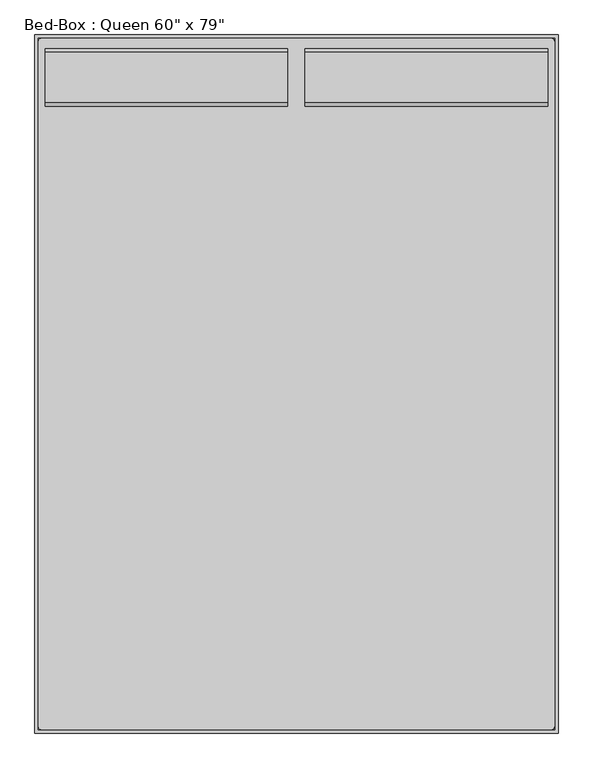
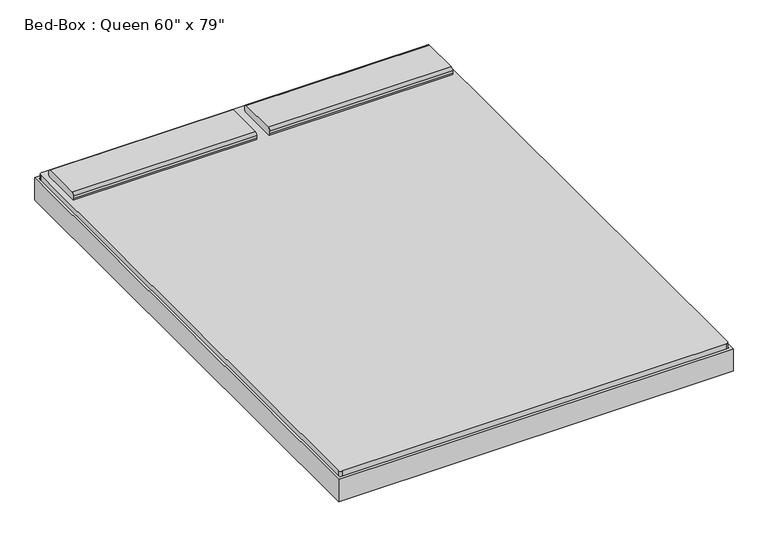
"""IFC4 building model written with IfcOpenShell, lengths in millimetres: furniture geometry."""

from ifc_helpers import new_model, si_unit, point, frame, frame_2d, origin, place, context, project, spatial, polyline, circle_curve, trimmed, segment, composite_curve, outline, extrude, source, transform, mapped, element, save
from ifc_brep_helpers import plane_surface, cylinder_surface, revolved_surface, advanced_brep


def furniture_0647d374(model_context):
    return source(origin(), model_context, "Body", "SolidModel", [
        advanced_brep(
        [(-1540.447541, -2469.6295082, 196.85), (-1540.447541, -2469.6295082, 177.8), (-1540.447541, -2545.8295082, 177.8), (-1540.447541, -2545.8295082, 196.85), (-1477.5113525, -2469.6295082, 196.85), (-1489.647541, -2469.6295082, 177.8), (-1489.647541, -2545.8295082, 177.8), (-1477.5113525, -2545.8295082, 196.85), (-1396.3115092, -2469.6295082, 22.716374), (-1413.5766725, -2469.6295082, 14.6654962), (-1413.5766725, -2545.8295082, 14.6654962), (-1396.3115092, -2545.8295082, 22.716374), (-1390.5564547, -2469.6295082, 0.0), (-1390.5564547, -2469.6295082, 19.05), (-1390.5564547, -2545.8295082, 0.0), (-1390.5564547, -2545.8295082, 19.05), (-1311.9439489, -2469.6295082, 19.05), (-1311.9439489, -2469.6295082, 0.0), (-1311.9439489, -2545.8295082, 0.0), (-1311.9439489, -2545.8295082, 19.05), (-1299.2439489, -2469.6295082, 3.4029547), (-1308.7689489, -2469.6295082, 19.9007387), (-1299.2439489, -2545.8295082, 3.4029547), (-1308.7689489, -2545.8295082, 19.9007387), (-1244.2513357, -2469.6295082, 57.15), (-1239.1469036, -2469.6295082, 38.1), (-1239.1469036, -2545.8295082, 38.1), (-1244.2513357, -2545.8295082, 57.15), (1922.5562537, -2469.6295082, 57.15), (1917.4518216, -2469.6295082, 38.1), (1917.4518216, -2545.8295082, 38.1), (1922.5562537, -2545.8295082, 57.15), (1987.0738669, -2469.6295082, 19.9007387), (1977.5488669, -2469.6295082, 3.4029547), (1977.5488669, -2545.8295082, 3.4029547), (1987.0738669, -2545.8295082, 19.9007387), (1990.2488669, -2469.6295082, 0.0), (1990.2488669, -2469.6295082, 19.05), (1990.2488669, -2545.8295082, 0.0), (1990.2488669, -2545.8295082, 19.05), (2068.8613728, -2469.6295082, 19.05), (2068.8613728, -2469.6295082, 0.0), (2068.8613728, -2545.8295082, 0.0), (2068.8613728, -2545.8295082, 19.05), (2091.8815906, -2469.6295082, 14.6654962), (2074.6164272, -2469.6295082, 22.716374), (2091.8815906, -2545.8295082, 14.6654962), (2074.6164272, -2545.8295082, 22.716374), (2155.8162705, -2469.6295082, 196.85), (2167.952459, -2469.6295082, 177.8), (2167.952459, -2545.8295082, 177.8), (2155.8162705, -2545.8295082, 196.85), (2218.752459, -2469.6295082, 196.85), (2218.752459, -2545.8295082, 196.85), (2218.752459, -2545.8295082, 177.8), (2218.752459, -2469.6295082, 177.8)],
        [
            (0, 1),
            (1, 2),
            (2, 3),
            (3, 0),
            (0, 4),
            (4, 5),
            (5, 1),
            (5, 6),
            (6, 2),
            (6, 7),
            (7, 3),
            (7, 4),
            (4, 8),
            (8, 9),
            (9, 5),
            (9, 10),
            (10, 6),
            (10, 11),
            (11, 7),
            (11, 8),
            (12, 9, circle_curve(frame((-1390.5564547, -2469.6295082, 25.4), z_axis=(0.0, 1.0, 0.0), x_axis=(-0.906307787036663, 0.0, -0.4226182617406713)), 25.4)),
            (8, 13, circle_curve(frame((-1390.5564547, -2469.6295082, 25.4), z_axis=(0.0, -1.0, 0.0), x_axis=(-0.906307787036663, 0.0, -0.4226182617406713)), 6.35)),
            (13, 12),
            (14, 10, circle_curve(frame((-1390.5564547, -2545.8295082, 25.4), z_axis=(0.0, 1.0, 0.0), x_axis=(-0.906307787036663, 0.0, -0.4226182617406713)), 25.4)),
            (12, 14),
            (15, 11, circle_curve(frame((-1390.5564547, -2545.8295082, 25.4), z_axis=(0.0, 1.0, 0.0), x_axis=(-0.906307787036663, 0.0, -0.4226182617406713)), 6.35)),
            (14, 15),
            (15, 13),
            (13, 16),
            (16, 17),
            (17, 12),
            (17, 18),
            (18, 14),
            (18, 19),
            (19, 15),
            (19, 16),
            (20, 17, circle_curve(frame((-1311.9439489, -2469.6295082, 25.4), z_axis=(0.0, 1.0, 0.0), x_axis=(0.0, 0.0, -1.0)), 25.4)),
            (16, 21, circle_curve(frame((-1311.9439489, -2469.6295082, 25.4), z_axis=(0.0, -1.0, 0.0), x_axis=(0.0, 0.0, -1.0)), 6.35)),
            (21, 20),
            (22, 18, circle_curve(frame((-1311.9439489, -2545.8295082, 25.4), z_axis=(0.0, 1.0, 0.0), x_axis=(0.0, 0.0, -1.0)), 25.4)),
            (20, 22),
            (23, 19, circle_curve(frame((-1311.9439489, -2545.8295082, 25.4), z_axis=(0.0, 1.0, 0.0), x_axis=(0.0, 0.0, -1.0)), 6.35)),
            (22, 23),
            (23, 21),
            (21, 24),
            (24, 25),
            (25, 20),
            (25, 26),
            (26, 22),
            (26, 27),
            (27, 23),
            (27, 24),
            (24, 28),
            (28, 29),
            (29, 25),
            (29, 30),
            (30, 26),
            (30, 31),
            (31, 27),
            (31, 28),
            (28, 32),
            (32, 33),
            (33, 29),
            (33, 34),
            (34, 30),
            (34, 35),
            (35, 31),
            (35, 32),
            (36, 33, circle_curve(frame((1990.2488669, -2469.6295082, 25.4), z_axis=(0.0, 1.0, 0.0), x_axis=(-0.5000000000000479, 0.0, -0.866025403784411)), 25.4)),
            (32, 37, circle_curve(frame((1990.2488669, -2469.6295082, 25.4), z_axis=(0.0, -1.0, 0.0), x_axis=(-0.5000000000000479, 0.0, -0.866025403784411)), 6.35)),
            (37, 36),
            (38, 34, circle_curve(frame((1990.2488669, -2545.8295082, 25.4), z_axis=(0.0, 1.0, 0.0), x_axis=(-0.5000000000000479, 0.0, -0.866025403784411)), 25.4)),
            (36, 38),
            (39, 35, circle_curve(frame((1990.2488669, -2545.8295082, 25.4), z_axis=(0.0, 1.0, 0.0), x_axis=(-0.5000000000000479, 0.0, -0.866025403784411)), 6.35)),
            (38, 39),
            (39, 37),
            (37, 40),
            (40, 41),
            (41, 36),
            (41, 42),
            (42, 38),
            (42, 43),
            (43, 39),
            (43, 40),
            (44, 41, circle_curve(frame((2068.8613728, -2469.6295082, 25.4), z_axis=(0.0, 1.0, 0.0), x_axis=(0.0, 0.0, -1.0)), 25.4)),
            (40, 45, circle_curve(frame((2068.8613728, -2469.6295082, 25.4), z_axis=(0.0, -1.0, 0.0), x_axis=(0.0, 0.0, -1.0)), 6.35)),
            (45, 44),
            (46, 42, circle_curve(frame((2068.8613728, -2545.8295082, 25.4), z_axis=(0.0, 1.0, 0.0), x_axis=(0.0, 0.0, -1.0)), 25.4)),
            (44, 46),
            (47, 43, circle_curve(frame((2068.8613728, -2545.8295082, 25.4), z_axis=(0.0, 1.0, 0.0), x_axis=(0.0, 0.0, -1.0)), 6.35)),
            (46, 47),
            (47, 45),
            (45, 48),
            (48, 49),
            (49, 44),
            (49, 50),
            (50, 46),
            (50, 51),
            (51, 47),
            (51, 48),
            (52, 53),
            (53, 54),
            (54, 55),
            (55, 52),
            (48, 52),
            (55, 49),
            (54, 50),
            (53, 51),
        ],
        [
            plane_surface(frame((-1540.447541, -2774.4295082, -127.5947323), z_axis=(-1.0, 0.0, 0.0), x_axis=(0.0, 1.0, 0.0))),
            plane_surface(frame((-1540.447541, -2469.6295082, 196.85), z_axis=(0.0, 1.0, 0.0), x_axis=(1.0, 0.0, 0.0))),
            plane_surface(frame((-1540.447541, -2469.6295082, 177.8), z_axis=(0.0, 0.0, -1.0), x_axis=(1.0, 0.0, 0.0))),
            plane_surface(frame((-1540.447541, -2545.8295082, 177.8), z_axis=(0.0, -1.0, 0.0), x_axis=(1.0, 0.0, 0.0))),
            plane_surface(frame((-1540.447541, -2545.8295082, 196.85), z_axis=(0.0, 0.0, 1.0), x_axis=(1.0, 0.0, 0.0))),
            plane_surface(frame((-1477.5113525, -2469.6295082, 196.85), z_axis=(0.0, 1.0, 0.0), x_axis=(0.42261826174067096, 0.0, -0.9063077870366633))),
            plane_surface(frame((-1489.647541, -2469.6295082, 177.8), z_axis=(-0.9063077870366629, 0.0, -0.4226182617406717), x_axis=(0.4226182617406717, 0.0, -0.9063077870366629))),
            plane_surface(frame((-1489.647541, -2545.8295082, 177.8), z_axis=(0.0, -1.0, 0.0), x_axis=(0.4226182617406704, 0.0, -0.9063077870366635))),
            plane_surface(frame((-1477.5113525, -2545.8295082, 196.85), z_axis=(0.906307787036663, 0.0, 0.42261826174067146), x_axis=(0.42261826174067146, 0.0, -0.906307787036663))),
            plane_surface(frame((-1390.5564547, -2469.6295082, 25.4), z_axis=(0.0, 1.0, 0.0), x_axis=(-0.906307787036663, 0.0, -0.4226182617406713))),
            cylinder_surface(frame((-1390.5564547, -2774.4295082, 25.4), z_axis=(0.0, -1.0, 0.0), x_axis=(-0.906307787036663, 0.0, -0.4226182617406713)), 25.4),
            plane_surface(frame((-1390.5564547, -2545.8295082, 25.4), z_axis=(0.0, -1.0, 0.0), x_axis=(-0.906307787036663, 0.0, -0.4226182617406713))),
            revolved_surface(polyline([(-1396.3115091476827, -2545.8295082, 22.716374037946736), (-1396.3115091476827, -2469.6295082, 22.716374037946736)]), (-1390.5564547, -2774.4295082, 25.4), (0.0, -1.0, 0.0)),
            plane_surface(frame((-1390.5564547, -2469.6295082, 19.05), z_axis=(0.0, 1.0, 0.0), x_axis=(1.0, 0.0, 0.0))),
            plane_surface(frame((-1390.5564547, -2469.6295082, 0.0), z_axis=(0.0, 0.0, -1.0), x_axis=(1.0, 0.0, 0.0))),
            plane_surface(frame((-1390.5564547, -2545.8295082, 0.0), z_axis=(0.0, -1.0, 0.0), x_axis=(1.0, 0.0, 0.0))),
            plane_surface(frame((-1390.5564547, -2545.8295082, 19.05), z_axis=(0.0, 0.0, 1.0), x_axis=(1.0, 0.0, 0.0))),
            plane_surface(frame((-1311.9439489, -2469.6295082, 25.4), z_axis=(0.0, 1.0, 0.0), x_axis=(0.0, 0.0, -1.0))),
            cylinder_surface(frame((-1311.9439489, -2774.4295082, 25.4), z_axis=(0.0, -1.0, 0.0), x_axis=(0.0, 0.0, -1.0)), 25.4),
            plane_surface(frame((-1311.9439489, -2545.8295082, 25.4), z_axis=(0.0, -1.0, 0.0), x_axis=(0.0, 0.0, -1.0))),
            revolved_surface(polyline([(-1311.9439489, -2545.8295082, 19.049999999999997), (-1311.9439489, -2469.6295082, 19.049999999999997)]), (-1311.9439489, -2774.4295082, 25.4), (0.0, -1.0, 0.0)),
            plane_surface(frame((-1308.7689489, -2469.6295082, 19.9007387), z_axis=(0.0, 1.0000000000000002, 0.0), x_axis=(0.8660254037844785, 0.0, 0.4999999999999312))),
            plane_surface(frame((-1299.2439489, -2469.6295082, 3.4029547), z_axis=(0.49999999999993033, 0.0, -0.8660254037844789), x_axis=(0.8660254037844789, 0.0, 0.49999999999993033))),
            plane_surface(frame((-1299.2439489, -2545.8295082, 3.4029547), z_axis=(0.0, -1.0, 0.0), x_axis=(0.8660254037844797, 0.0, 0.4999999999999289))),
            plane_surface(frame((-1308.7689489, -2545.8295082, 19.9007387), z_axis=(-0.4999999999999325, 0.0, 0.8660254037844777), x_axis=(0.8660254037844777, 0.0, 0.4999999999999325))),
            plane_surface(frame((-1244.2513357, -2469.6295082, 57.15), z_axis=(0.0, 1.0, 0.0), x_axis=(1.0, 0.0, 0.0))),
            plane_surface(frame((-1239.1469036, -2469.6295082, 38.1), z_axis=(0.0, 0.0, -1.0), x_axis=(1.0, 0.0, 0.0))),
            plane_surface(frame((-1239.1469036, -2545.8295082, 38.1), z_axis=(0.0, -1.0, 0.0), x_axis=(1.0, 0.0, 0.0))),
            plane_surface(frame((-1244.2513357, -2545.8295082, 57.15), z_axis=(0.0, 0.0, 1.0), x_axis=(1.0, 0.0, 0.0))),
            plane_surface(frame((1922.5562537, -2469.6295082, 57.15), z_axis=(0.0, 1.0, 0.0), x_axis=(0.86602540378441, 0.0, -0.5000000000000497))),
            plane_surface(frame((1917.4518216, -2469.6295082, 38.1), z_axis=(-0.5000000000000524, 0.0, -0.8660254037844084), x_axis=(0.8660254037844084, 0.0, -0.5000000000000524))),
            plane_surface(frame((1917.4518216, -2545.8295082, 38.1), z_axis=(0.0, -1.0, 0.0), x_axis=(0.8660254037844108, 0.0, -0.5000000000000483))),
            plane_surface(frame((1922.5562537, -2545.8295082, 57.15), z_axis=(0.500000000000048, 0.0, 0.866025403784411), x_axis=(0.866025403784411, 0.0, -0.500000000000048))),
            plane_surface(frame((1990.2488669, -2469.6295082, 25.4), z_axis=(0.0, 1.0000000000000002, 0.0), x_axis=(-0.500000000000048, 0.0, -0.8660254037844111))),
            cylinder_surface(frame((1990.2488669, -2774.4295082, 25.4), z_axis=(0.0, -1.0, 0.0), x_axis=(-0.5000000000000479, 0.0, -0.866025403784411)), 25.4),
            plane_surface(frame((1990.2488669, -2545.8295082, 25.4), z_axis=(0.0, -1.0000000000000002, 0.0), x_axis=(-0.500000000000048, 0.0, -0.8660254037844111))),
            revolved_surface(polyline([(1987.0738668999995, -2545.8295082, 19.90073868596899), (1987.0738668999995, -2469.6295082, 19.90073868596899)]), (1990.2488669, -2774.4295082, 25.4), (0.0, -1.0, 0.0)),
            plane_surface(frame((1990.2488669, -2469.6295082, 19.05), z_axis=(0.0, 1.0, 0.0), x_axis=(1.0, 0.0, 0.0))),
            plane_surface(frame((1990.2488669, -2469.6295082, 0.0), z_axis=(0.0, 0.0, -1.0), x_axis=(1.0, 0.0, 0.0))),
            plane_surface(frame((1990.2488669, -2545.8295082, 0.0), z_axis=(0.0, -1.0, 0.0), x_axis=(1.0, 0.0, 0.0))),
            plane_surface(frame((1990.2488669, -2545.8295082, 19.05), z_axis=(0.0, 0.0, 1.0), x_axis=(1.0, 0.0, 0.0))),
            plane_surface(frame((2068.8613728, -2469.6295082, 25.4), z_axis=(0.0, 1.0, 0.0), x_axis=(0.0, 0.0, -1.0))),
            cylinder_surface(frame((2068.8613728, -2774.4295082, 25.4), z_axis=(0.0, -1.0, 0.0), x_axis=(0.0, 0.0, -1.0)), 25.4),
            plane_surface(frame((2068.8613728, -2545.8295082, 25.4), z_axis=(0.0, -1.0, 0.0), x_axis=(0.0, 0.0, -1.0))),
            revolved_surface(polyline([(2068.8613728, -2545.8295082, 19.049999999999997), (2068.8613728, -2469.6295082, 19.049999999999997)]), (2068.8613728, -2774.4295082, 25.4), (0.0, -1.0, 0.0)),
            plane_surface(frame((2074.6164272, -2469.6295082, 22.716374), z_axis=(0.0, 1.0, 0.0), x_axis=(0.4226182617405407, 0.0, 0.906307787036724))),
            plane_surface(frame((2091.8815906, -2469.6295082, 14.6654962), z_axis=(0.9063077870367238, 0.0, -0.4226182617405412), x_axis=(0.4226182617405412, 0.0, 0.9063077870367238))),
            plane_surface(frame((2091.8815906, -2545.8295082, 14.6654962), z_axis=(0.0, -1.0000000000000002, 0.0), x_axis=(0.422618261740542, 0.0, 0.9063077870367234))),
            plane_surface(frame((2074.6164272, -2545.8295082, 22.716374), z_axis=(-0.9063077870367237, 0.0, 0.4226182617405417), x_axis=(0.4226182617405417, 0.0, 0.9063077870367237))),
            plane_surface(frame((2218.752459, -2774.4295082, -127.5947323), z_axis=(1.0, 0.0, 0.0), x_axis=(0.0, 1.0, 0.0))),
            plane_surface(frame((2155.8162705, -2469.6295082, 196.85), z_axis=(0.0, 1.0, 0.0), x_axis=(1.0, 0.0, 0.0))),
            plane_surface(frame((2167.952459, -2469.6295082, 177.8), z_axis=(0.0, 0.0, -1.0), x_axis=(1.0, 0.0, 0.0))),
            plane_surface(frame((2167.952459, -2545.8295082, 177.8), z_axis=(0.0, -1.0, 0.0), x_axis=(1.0, 0.0, 0.0))),
            plane_surface(frame((2155.8162705, -2545.8295082, 196.85), z_axis=(0.0, 0.0, 1.0), x_axis=(1.0, 0.0, 0.0))),
        ],
        [
            (0, [[1, 2, 3, 4]]),
            (1, [[-1, 5, 6, 7]]),
            (2, [[-2, -7, 8, 9]]),
            (3, [[-3, -9, 10, 11]]),
            (4, [[-4, -11, 12, -5]]),
            (5, [[-6, 13, 14, 15]]),
            (6, [[-8, -15, 16, 17]]),
            (7, [[-10, -17, 18, 19]]),
            (8, [[-12, -19, 20, -13]]),
            (9, [[21, -14, 22, 23]]),
            (10, [[24, -16, -21, 25]]),
            (11, [[26, -18, -24, 27]]),
            (12, [[-22, -20, -26, 28]]),
            (13, [[-23, 29, 30, 31]]),
            (14, [[-25, -31, 32, 33]]),
            (15, [[-27, -33, 34, 35]]),
            (16, [[-28, -35, 36, -29]]),
            (17, [[37, -30, 38, 39]]),
            (18, [[40, -32, -37, 41]]),
            (19, [[42, -34, -40, 43]]),
            (20, [[-38, -36, -42, 44]]),
            (21, [[-39, 45, 46, 47]]),
            (22, [[-41, -47, 48, 49]]),
            (23, [[-43, -49, 50, 51]]),
            (24, [[-44, -51, 52, -45]]),
            (25, [[-46, 53, 54, 55]]),
            (26, [[-48, -55, 56, 57]]),
            (27, [[-50, -57, 58, 59]]),
            (28, [[-52, -59, 60, -53]]),
            (29, [[-54, 61, 62, 63]]),
            (30, [[-56, -63, 64, 65]]),
            (31, [[-58, -65, 66, 67]]),
            (32, [[-60, -67, 68, -61]]),
            (33, [[69, -62, 70, 71]]),
            (34, [[72, -64, -69, 73]]),
            (35, [[74, -66, -72, 75]]),
            (36, [[-70, -68, -74, 76]]),
            (37, [[-71, 77, 78, 79]]),
            (38, [[-73, -79, 80, 81]]),
            (39, [[-75, -81, 82, 83]]),
            (40, [[-76, -83, 84, -77]]),
            (41, [[85, -78, 86, 87]]),
            (42, [[88, -80, -85, 89]]),
            (43, [[90, -82, -88, 91]]),
            (44, [[-86, -84, -90, 92]]),
            (45, [[-87, 93, 94, 95]]),
            (46, [[-89, -95, 96, 97]]),
            (47, [[-91, -97, 98, 99]]),
            (48, [[-92, -99, 100, -93]]),
            (49, [[101, 102, 103, 104]]),
            (50, [[-94, 105, -104, 106]]),
            (51, [[-96, -106, -103, 107]]),
            (52, [[-98, -107, -102, 108]]),
            (53, [[-100, -108, -101, -105]]),
        ],
    ),
        extrude(outline(composite_curve([segment(polyline([(-1515.047541, 2280.1704918), (2193.352459, 2280.1704918)]), True, "CONTINUOUS"), segment(trimmed(circle_curve(frame_2d((2193.352459, 2254.7704918)), 25.4), [point((2193.352459, 2280.1704918))], [point((2218.752459, 2254.7704918))], False, "CARTESIAN"), True, "CONTINUOUS"), segment(polyline([(2218.752459, 2254.7704918), (2218.752459, -2723.6295082)]), True, "CONTINUOUS"), segment(trimmed(circle_curve(frame_2d((2193.352459, -2723.6295082)), 25.4), [point((2218.752459, -2723.6295082))], [point((2193.352459, -2749.0295082))], False, "CARTESIAN"), True, "CONTINUOUS"), segment(polyline([(2193.352459, -2749.0295082), (-1515.047541, -2749.0295082)]), True, "CONTINUOUS"), segment(trimmed(circle_curve(frame_2d((-1515.047541, -2723.6295082)), 25.4), [point((-1515.047541, -2749.0295082))], [point((-1540.447541, -2723.6295082))], False, "CARTESIAN"), True, "CONTINUOUS"), segment(polyline([(-1540.447541, -2723.6295082), (-1540.447541, 2254.7704918)]), True, "CONTINUOUS"), segment(trimmed(circle_curve(frame_2d((-1515.047541, 2254.7704918)), 25.4), [point((-1540.447541, 2254.7704918))], [point((-1515.047541, 2280.1704918))], False, "CARTESIAN"), True, "CONTINUOUS")], self_intersect=False)), frame((0.0, 0.0, 203.2), z_axis=(0.0, 0.0, 1.0), x_axis=(1.0, 0.0, 0.0)), (0.0, 0.0, 1.0), 203.2),
        advanced_brep(
        [(-1540.1231784, 2051.5704918, 177.8), (-1540.1231784, 1975.3704918, 177.8), (-1540.1231784, 1975.3704918, 196.85), (-1540.1231784, 2051.5704918, 196.85), (-1489.3231784, 2051.5704918, 177.8), (-1489.3231784, 1975.3704918, 177.8), (-1477.1869899, 1975.3704918, 196.85), (-1477.1869899, 2051.5704918, 196.85), (-1413.2523099, 2051.5704918, 14.6654962), (-1413.2523099, 1975.3704918, 14.6654962), (-1395.9871466, 1975.3704918, 22.716374), (-1395.9871466, 2051.5704918, 22.716374), (-1390.2320921, 1975.3704918, 0.0), (-1390.2320921, 2051.5704918, 0.0), (-1390.2320921, 1975.3704918, 19.05), (-1390.2320921, 2051.5704918, 19.05), (-1311.6195862, 2051.5704918, 0.0), (-1311.6195862, 1975.3704918, 0.0), (-1311.6195862, 1975.3704918, 19.05), (-1311.6195862, 2051.5704918, 19.05), (-1298.9195862, 1975.3704918, 3.4029547), (-1298.9195862, 2051.5704918, 3.4029547), (-1308.4445862, 1975.3704918, 19.9007387), (-1308.4445862, 2051.5704918, 19.9007387), (-1238.822541, 2051.5704918, 38.1), (-1238.822541, 1975.3704918, 38.1), (-1243.9269731, 1975.3704918, 57.15), (-1243.9269731, 2051.5704918, 57.15), (1917.4518216, 2051.5704918, 38.1), (1917.4518216, 1975.3704918, 38.1), (1922.5562537, 1975.3704918, 57.15), (1922.5562537, 2051.5704918, 57.15), (1977.5488669, 2051.5704918, 3.4029547), (1977.5488669, 1975.3704918, 3.4029547), (1987.0738669, 1975.3704918, 19.9007387), (1987.0738669, 2051.5704918, 19.9007387), (1990.2488669, 1975.3704918, 0.0), (1990.2488669, 2051.5704918, 0.0), (1990.2488669, 1975.3704918, 19.05), (1990.2488669, 2051.5704918, 19.05), (2068.8613728, 2051.5704918, 0.0), (2068.8613728, 1975.3704918, 0.0), (2068.8613728, 1975.3704918, 19.05), (2068.8613728, 2051.5704918, 19.05), (2091.8815906, 1975.3704918, 14.6654962), (2091.8815906, 2051.5704918, 14.6654962), (2074.6164272, 1975.3704918, 22.716374), (2074.6164272, 2051.5704918, 22.716374), (2167.952459, 2051.5704918, 177.8), (2167.952459, 1975.3704918, 177.8), (2155.8162705, 1975.3704918, 196.85), (2155.8162705, 2051.5704918, 196.85), (2218.752459, 2051.5704918, 177.8), (2218.752459, 2051.5704918, 196.85), (2218.752459, 1975.3704918, 196.85), (2218.752459, 1975.3704918, 177.8)],
        [
            (0, 1),
            (1, 2),
            (2, 3),
            (3, 0),
            (0, 4),
            (4, 5),
            (5, 1),
            (5, 6),
            (6, 2),
            (6, 7),
            (7, 3),
            (7, 4),
            (4, 8),
            (8, 9),
            (9, 5),
            (9, 10),
            (10, 6),
            (10, 11),
            (11, 7),
            (11, 8),
            (12, 9, circle_curve(frame((-1390.2320921, 1975.3704918, 25.4), z_axis=(0.0, 1.0, 0.0), x_axis=(-0.9063077870366486, 0.0, -0.42261826174070233)), 25.4)),
            (8, 13, circle_curve(frame((-1390.2320921, 2051.5704918, 25.4), z_axis=(0.0, -1.0, 0.0), x_axis=(-0.9063077870366486, 0.0, -0.42261826174070233)), 25.4)),
            (13, 12),
            (14, 10, circle_curve(frame((-1390.2320921, 1975.3704918, 25.4), z_axis=(0.0, 1.0, 0.0), x_axis=(-0.9063077870366486, 0.0, -0.42261826174070233)), 6.35)),
            (12, 14),
            (15, 11, circle_curve(frame((-1390.2320921, 2051.5704918, 25.4), z_axis=(0.0, 1.0, 0.0), x_axis=(-0.9063077870366486, 0.0, -0.42261826174070233)), 6.35)),
            (14, 15),
            (15, 13),
            (13, 16),
            (16, 17),
            (17, 12),
            (17, 18),
            (18, 14),
            (18, 19),
            (19, 15),
            (19, 16),
            (20, 17, circle_curve(frame((-1311.6195862, 1975.3704918, 25.4), z_axis=(0.0, 1.0, 0.0), x_axis=(0.0, 0.0, -1.0)), 25.4)),
            (16, 21, circle_curve(frame((-1311.6195862, 2051.5704918, 25.4), z_axis=(0.0, -1.0, 0.0), x_axis=(0.0, 0.0, -1.0)), 25.4)),
            (21, 20),
            (22, 18, circle_curve(frame((-1311.6195862, 1975.3704918, 25.4), z_axis=(0.0, 1.0, 0.0), x_axis=(0.0, 0.0, -1.0)), 6.35)),
            (20, 22),
            (23, 19, circle_curve(frame((-1311.6195862, 2051.5704918, 25.4), z_axis=(0.0, 1.0, 0.0), x_axis=(0.0, 0.0, -1.0)), 6.35)),
            (22, 23),
            (23, 21),
            (21, 24),
            (24, 25),
            (25, 20),
            (25, 26),
            (26, 22),
            (26, 27),
            (27, 23),
            (27, 24),
            (24, 28),
            (28, 29),
            (29, 25),
            (29, 30),
            (30, 26),
            (30, 31),
            (31, 27),
            (31, 28),
            (28, 32),
            (32, 33),
            (33, 29),
            (33, 34),
            (34, 30),
            (34, 35),
            (35, 31),
            (35, 32),
            (36, 33, circle_curve(frame((1990.2488669, 1975.3704918, 25.4), z_axis=(0.0, 1.0, 0.0), x_axis=(-0.5000000000000463, 0.0, -0.8660254037844118)), 25.4)),
            (32, 37, circle_curve(frame((1990.2488669, 2051.5704918, 25.4), z_axis=(0.0, -1.0, 0.0), x_axis=(-0.5000000000000463, 0.0, -0.8660254037844118)), 25.4)),
            (37, 36),
            (38, 34, circle_curve(frame((1990.2488669, 1975.3704918, 25.4), z_axis=(0.0, 1.0, 0.0), x_axis=(-0.5000000000000463, 0.0, -0.8660254037844118)), 6.35)),
            (36, 38),
            (39, 35, circle_curve(frame((1990.2488669, 2051.5704918, 25.4), z_axis=(0.0, 1.0, 0.0), x_axis=(-0.5000000000000463, 0.0, -0.8660254037844118)), 6.35)),
            (38, 39),
            (39, 37),
            (37, 40),
            (40, 41),
            (41, 36),
            (41, 42),
            (42, 38),
            (42, 43),
            (43, 39),
            (43, 40),
            (44, 41, circle_curve(frame((2068.8613728, 1975.3704918, 25.4), z_axis=(0.0, 1.0, 0.0), x_axis=(0.0, 0.0, -1.0)), 25.4)),
            (40, 45, circle_curve(frame((2068.8613728, 2051.5704918, 25.4), z_axis=(0.0, -1.0, 0.0), x_axis=(0.0, 0.0, -1.0)), 25.4)),
            (45, 44),
            (46, 42, circle_curve(frame((2068.8613728, 1975.3704918, 25.4), z_axis=(0.0, 1.0, 0.0), x_axis=(0.0, 0.0, -1.0)), 6.35)),
            (44, 46),
            (47, 43, circle_curve(frame((2068.8613728, 2051.5704918, 25.4), z_axis=(0.0, 1.0, 0.0), x_axis=(0.0, 0.0, -1.0)), 6.35)),
            (46, 47),
            (47, 45),
            (45, 48),
            (48, 49),
            (49, 44),
            (49, 50),
            (50, 46),
            (50, 51),
            (51, 47),
            (51, 48),
            (52, 53),
            (53, 54),
            (54, 55),
            (55, 52),
            (48, 52),
            (55, 49),
            (54, 50),
            (53, 51),
        ],
        [
            plane_surface(frame((-1540.1231784, 2305.5704918, -152.9490627), z_axis=(-1.0, 0.0, 0.0), x_axis=(0.0, 1.0, 0.0))),
            plane_surface(frame((-1540.1231784, 2051.5704918, 177.8), z_axis=(0.0, 0.0, -1.0), x_axis=(1.0, 0.0, 0.0))),
            plane_surface(frame((-1540.1231784, 1975.3704918, 177.8), z_axis=(0.0, -1.0, 0.0), x_axis=(1.0, 0.0, 0.0))),
            plane_surface(frame((-1540.1231784, 1975.3704918, 196.85), z_axis=(0.0, 0.0, 1.0), x_axis=(1.0, 0.0, 0.0))),
            plane_surface(frame((-1540.1231784, 2051.5704918, 196.85), z_axis=(0.0, 1.0, 0.0), x_axis=(1.0, 0.0, 0.0))),
            plane_surface(frame((-1489.3231784, 2051.5704918, 177.8), z_axis=(-0.906307787036649, 0.0, -0.42261826174070155), x_axis=(0.42261826174070155, 0.0, -0.906307787036649))),
            plane_surface(frame((-1489.3231784, 1975.3704918, 177.8), z_axis=(0.0, -1.0, 0.0), x_axis=(0.42261826174070133, 0.0, -0.9063077870366492))),
            plane_surface(frame((-1477.1869899, 1975.3704918, 196.85), z_axis=(0.9063077870366489, 0.0, 0.4226182617407018), x_axis=(0.4226182617407018, 0.0, -0.9063077870366489))),
            plane_surface(frame((-1477.1869899, 2051.5704918, 196.85), z_axis=(0.0, 1.0, 0.0), x_axis=(0.4226182617407019, 0.0, -0.9063077870366488))),
            cylinder_surface(frame((-1390.2320921, 2305.5704918, 25.4), z_axis=(0.0, -1.0, 0.0), x_axis=(-0.9063077870366486, 0.0, -0.42261826174070233)), 25.4),
            plane_surface(frame((-1390.2320921, 1975.3704918, 25.4), z_axis=(0.0, -1.0, 0.0), x_axis=(-0.9063077870366486, 0.0, -0.42261826174070233))),
            revolved_surface(polyline([(-1395.9871465476829, 1975.3704918, 22.71637403794654), (-1395.9871465476829, 2051.5704918, 22.71637403794654)]), (-1390.2320921, 2305.5704918, 25.4), (0.0, -1.0, 0.0)),
            plane_surface(frame((-1390.2320921, 2051.5704918, 25.4), z_axis=(0.0, 1.0, 0.0), x_axis=(-0.9063077870366486, 0.0, -0.42261826174070233))),
            plane_surface(frame((-1390.2320921, 2051.5704918, 0.0), z_axis=(0.0, 0.0, -1.0), x_axis=(1.0, 0.0, 0.0))),
            plane_surface(frame((-1390.2320921, 1975.3704918, 0.0), z_axis=(0.0, -1.0, 0.0), x_axis=(1.0, 0.0, 0.0))),
            plane_surface(frame((-1390.2320921, 1975.3704918, 19.05), z_axis=(0.0, 0.0, 1.0), x_axis=(1.0, 0.0, 0.0))),
            plane_surface(frame((-1390.2320921, 2051.5704918, 19.05), z_axis=(0.0, 1.0, 0.0), x_axis=(1.0, 0.0, 0.0))),
            cylinder_surface(frame((-1311.6195862, 2305.5704918, 25.4), z_axis=(0.0, -1.0, 0.0), x_axis=(0.0, 0.0, -1.0)), 25.4),
            plane_surface(frame((-1311.6195862, 1975.3704918, 25.4), z_axis=(0.0, -1.0, 0.0), x_axis=(0.0, 0.0, -1.0))),
            revolved_surface(polyline([(-1311.6195862, 1975.3704918, 19.049999999999997), (-1311.6195862, 2051.5704918, 19.049999999999997)]), (-1311.6195862, 2305.5704918, 25.4), (0.0, -1.0, 0.0)),
            plane_surface(frame((-1311.6195862, 2051.5704918, 25.4), z_axis=(0.0, 1.0, 0.0), x_axis=(0.0, 0.0, -1.0))),
            plane_surface(frame((-1298.9195862, 2051.5704918, 3.4029547), z_axis=(0.49999999999988004, 0.0, -0.866025403784508), x_axis=(0.866025403784508, 0.0, 0.49999999999988004))),
            plane_surface(frame((-1298.9195862, 1975.3704918, 3.4029547), z_axis=(0.0, -1.0, 0.0), x_axis=(0.8660254037845087, 0.0, 0.4999999999998787))),
            plane_surface(frame((-1308.4445862, 1975.3704918, 19.9007387), z_axis=(-0.49999999999987754, 0.0, 0.8660254037845093), x_axis=(0.8660254037845093, 0.0, 0.49999999999987754))),
            plane_surface(frame((-1308.4445862, 2051.5704918, 19.9007387), z_axis=(0.0, 1.0, 0.0), x_axis=(0.8660254037845093, 0.0, 0.49999999999987754))),
            plane_surface(frame((-1238.822541, 2051.5704918, 38.1), z_axis=(0.0, 0.0, -1.0), x_axis=(1.0, 0.0, 0.0))),
            plane_surface(frame((-1238.822541, 1975.3704918, 38.1), z_axis=(0.0, -1.0, 0.0), x_axis=(1.0, 0.0, 0.0))),
            plane_surface(frame((-1243.9269731, 1975.3704918, 57.15), z_axis=(0.0, 0.0, 1.0), x_axis=(1.0, 0.0, 0.0))),
            plane_surface(frame((-1243.9269731, 2051.5704918, 57.15), z_axis=(0.0, 1.0, 0.0), x_axis=(1.0, 0.0, 0.0))),
            plane_surface(frame((1917.4518216, 2051.5704918, 38.1), z_axis=(-0.500000000000042, 0.0, -0.8660254037844145), x_axis=(0.8660254037844145, 0.0, -0.500000000000042))),
            plane_surface(frame((1917.4518216, 1975.3704918, 38.1), z_axis=(0.0, -1.0000000000000002, 0.0), x_axis=(0.866025403784413, 0.0, -0.5000000000000447))),
            plane_surface(frame((1922.5562537, 1975.3704918, 57.15), z_axis=(0.5000000000000456, 0.0, 0.8660254037844124), x_axis=(0.8660254037844124, 0.0, -0.5000000000000456))),
            plane_surface(frame((1922.5562537, 2051.5704918, 57.15), z_axis=(0.0, 1.0, 0.0), x_axis=(0.8660254037844132, 0.0, -0.5000000000000442))),
            cylinder_surface(frame((1990.2488669, 2305.5704918, 25.4), z_axis=(0.0, -1.0, 0.0), x_axis=(-0.5000000000000463, 0.0, -0.8660254037844118)), 25.4),
            plane_surface(frame((1990.2488669, 1975.3704918, 25.4), z_axis=(0.0, -1.0000000000000002, 0.0), x_axis=(-0.5000000000000464, 0.0, -0.866025403784412))),
            revolved_surface(polyline([(1987.0738668999998, 1975.3704918, 19.90073868596898), (1987.0738668999998, 2051.5704918, 19.90073868596898)]), (1990.2488669, 2305.5704918, 25.4), (0.0, -1.0, 0.0)),
            plane_surface(frame((1990.2488669, 2051.5704918, 25.4), z_axis=(0.0, 1.0000000000000002, 0.0), x_axis=(-0.5000000000000464, 0.0, -0.866025403784412))),
            plane_surface(frame((1990.2488669, 2051.5704918, 0.0), z_axis=(0.0, 0.0, -1.0), x_axis=(1.0, 0.0, 0.0))),
            plane_surface(frame((1990.2488669, 1975.3704918, 0.0), z_axis=(0.0, -1.0, 0.0), x_axis=(1.0, 0.0, 0.0))),
            plane_surface(frame((1990.2488669, 1975.3704918, 19.05), z_axis=(0.0, 0.0, 1.0), x_axis=(1.0, 0.0, 0.0))),
            plane_surface(frame((1990.2488669, 2051.5704918, 19.05), z_axis=(0.0, 1.0, 0.0), x_axis=(1.0, 0.0, 0.0))),
            cylinder_surface(frame((2068.8613728, 2305.5704918, 25.4), z_axis=(0.0, -1.0, 0.0), x_axis=(0.0, 0.0, -1.0)), 25.4),
            plane_surface(frame((2068.8613728, 1975.3704918, 25.4), z_axis=(0.0, -1.0, 0.0), x_axis=(0.0, 0.0, -1.0))),
            revolved_surface(polyline([(2068.8613728, 1975.3704918, 19.049999999999997), (2068.8613728, 2051.5704918, 19.049999999999997)]), (2068.8613728, 2305.5704918, 25.4), (0.0, -1.0, 0.0)),
            plane_surface(frame((2068.8613728, 2051.5704918, 25.4), z_axis=(0.0, 1.0, 0.0), x_axis=(0.0, 0.0, -1.0))),
            plane_surface(frame((2091.8815906, 2051.5704918, 14.6654962), z_axis=(0.9063077870366797, 0.0, -0.42261826174063566), x_axis=(0.42261826174063566, 0.0, 0.9063077870366797))),
            plane_surface(frame((2091.8815906, 1975.3704918, 14.6654962), z_axis=(0.0, -1.0, 0.0), x_axis=(0.4226182617406362, 0.0, 0.9063077870366795))),
            plane_surface(frame((2074.6164272, 1975.3704918, 22.716374), z_axis=(-0.9063077870366798, 0.0, 0.42261826174063555), x_axis=(0.42261826174063555, 0.0, 0.9063077870366798))),
            plane_surface(frame((2074.6164272, 2051.5704918, 22.716374), z_axis=(0.0, 1.0000000000000002, 0.0), x_axis=(0.4226182617406349, 0.0, 0.9063077870366801))),
            plane_surface(frame((2218.752459, 2305.5704918, -152.9490627), z_axis=(1.0, 0.0, 0.0), x_axis=(0.0, 1.0, 0.0))),
            plane_surface(frame((2167.952459, 2051.5704918, 177.8), z_axis=(0.0, 0.0, -1.0), x_axis=(1.0, 0.0, 0.0))),
            plane_surface(frame((2167.952459, 1975.3704918, 177.8), z_axis=(0.0, -1.0, 0.0), x_axis=(1.0, 0.0, 0.0))),
            plane_surface(frame((2155.8162705, 1975.3704918, 196.85), z_axis=(0.0, 0.0, 1.0), x_axis=(1.0, 0.0, 0.0))),
            plane_surface(frame((2155.8162705, 2051.5704918, 196.85), z_axis=(0.0, 1.0, 0.0), x_axis=(1.0, 0.0, 0.0))),
        ],
        [
            (0, [[1, 2, 3, 4]]),
            (1, [[-1, 5, 6, 7]]),
            (2, [[-2, -7, 8, 9]]),
            (3, [[-3, -9, 10, 11]]),
            (4, [[-4, -11, 12, -5]]),
            (5, [[-6, 13, 14, 15]]),
            (6, [[-8, -15, 16, 17]]),
            (7, [[-10, -17, 18, 19]]),
            (8, [[-12, -19, 20, -13]]),
            (9, [[21, -14, 22, 23]]),
            (10, [[24, -16, -21, 25]]),
            (11, [[26, -18, -24, 27]]),
            (12, [[-22, -20, -26, 28]]),
            (13, [[-23, 29, 30, 31]]),
            (14, [[-25, -31, 32, 33]]),
            (15, [[-27, -33, 34, 35]]),
            (16, [[-28, -35, 36, -29]]),
            (17, [[37, -30, 38, 39]]),
            (18, [[40, -32, -37, 41]]),
            (19, [[42, -34, -40, 43]]),
            (20, [[-38, -36, -42, 44]]),
            (21, [[-39, 45, 46, 47]]),
            (22, [[-41, -47, 48, 49]]),
            (23, [[-43, -49, 50, 51]]),
            (24, [[-44, -51, 52, -45]]),
            (25, [[-46, 53, 54, 55]]),
            (26, [[-48, -55, 56, 57]]),
            (27, [[-50, -57, 58, 59]]),
            (28, [[-52, -59, 60, -53]]),
            (29, [[-54, 61, 62, 63]]),
            (30, [[-56, -63, 64, 65]]),
            (31, [[-58, -65, 66, 67]]),
            (32, [[-60, -67, 68, -61]]),
            (33, [[69, -62, 70, 71]]),
            (34, [[72, -64, -69, 73]]),
            (35, [[74, -66, -72, 75]]),
            (36, [[-70, -68, -74, 76]]),
            (37, [[-71, 77, 78, 79]]),
            (38, [[-73, -79, 80, 81]]),
            (39, [[-75, -81, 82, 83]]),
            (40, [[-76, -83, 84, -77]]),
            (41, [[85, -78, 86, 87]]),
            (42, [[88, -80, -85, 89]]),
            (43, [[90, -82, -88, 91]]),
            (44, [[-86, -84, -90, 92]]),
            (45, [[-87, 93, 94, 95]]),
            (46, [[-89, -95, 96, 97]]),
            (47, [[-91, -97, 98, 99]]),
            (48, [[-92, -99, 100, -93]]),
            (49, [[101, 102, 103, 104]]),
            (50, [[-94, 105, -104, 106]]),
            (51, [[-96, -106, -103, 107]]),
            (52, [[-98, -107, -102, 108]]),
            (53, [[-100, -108, -101, -105]]),
        ],
    ),
        extrude(outline(composite_curve([segment(polyline([(2178.5704918, 406.4), (1810.2704918, 406.4)]), True, "CONTINUOUS"), segment(trimmed(circle_curve(frame_2d((1810.2704918, 431.8)), 25.4), [point((1810.2704918, 406.4))], [point((1784.8704918, 431.8))], False, "CARTESIAN"), True, "CONTINUOUS"), segment(polyline([(1784.8704918, 431.8), (1784.8704918, 457.2)]), True, "CONTINUOUS"), segment(trimmed(circle_curve(frame_2d((1810.2704918, 457.2)), 25.4), [point((1784.8704918, 457.2))], [point((1810.2704918, 482.6))], False, "CARTESIAN"), True, "CONTINUOUS"), segment(polyline([(1810.2704918, 482.6), (2178.5704918, 482.6)]), True, "CONTINUOUS"), segment(trimmed(circle_curve(frame_2d((2178.5704918, 457.2)), 25.4), [point((2178.5704918, 482.6))], [point((2203.9704918, 457.2))], False, "CARTESIAN"), True, "CONTINUOUS"), segment(polyline([(2203.9704918, 457.2), (2203.9704918, 431.8)]), True, "CONTINUOUS"), segment(trimmed(circle_curve(frame_2d((2178.5704918, 431.8)), 25.4), [point((2203.9704918, 431.8))], [point((2178.5704918, 406.4))], False, "CARTESIAN"), True, "CONTINUOUS")], self_intersect=False)), frame((-1489.647541, 0.0, 0.0), z_axis=(1.0, 0.0, 0.0), x_axis=(0.0, 1.0, 0.0)), (0.0, 0.0, 1.0), 1765.3),
        extrude(outline(composite_curve([segment(polyline([(2178.5704918, 406.4), (1810.2704918, 406.4)]), True, "CONTINUOUS"), segment(trimmed(circle_curve(frame_2d((1810.2704918, 431.8)), 25.4), [point((1810.2704918, 406.4))], [point((1784.8704918, 431.8))], False, "CARTESIAN"), True, "CONTINUOUS"), segment(polyline([(1784.8704918, 431.8), (1784.8704918, 457.2)]), True, "CONTINUOUS"), segment(trimmed(circle_curve(frame_2d((1810.2704918, 457.2)), 25.4), [point((1784.8704918, 457.2))], [point((1810.2704918, 482.6))], False, "CARTESIAN"), True, "CONTINUOUS"), segment(polyline([(1810.2704918, 482.6), (2178.5704918, 482.6)]), True, "CONTINUOUS"), segment(trimmed(circle_curve(frame_2d((2178.5704918, 457.2)), 25.4), [point((2178.5704918, 482.6))], [point((2203.9704918, 457.2))], False, "CARTESIAN"), True, "CONTINUOUS"), segment(polyline([(2203.9704918, 457.2), (2203.9704918, 431.8)]), True, "CONTINUOUS"), segment(trimmed(circle_curve(frame_2d((2178.5704918, 431.8)), 25.4), [point((2203.9704918, 431.8))], [point((2178.5704918, 406.4))], False, "CARTESIAN"), True, "CONTINUOUS")], self_intersect=False)), frame((402.652459, 0.0, 0.0), z_axis=(1.0, 0.0, 0.0), x_axis=(0.0, 1.0, 0.0)), (0.0, 0.0, 1.0), 1765.3),
        extrude(outline(polyline([(2244.152459, 2305.5704918), (2244.152459, -2774.4295082), (-1565.847541, -2774.4295082), (-1565.847541, 2305.5704918), (2244.152459, 2305.5704918)]), holes=[polyline([(2218.752459, 2280.1704918), (-1540.447541, 2280.1704918), (-1540.447541, -2749.0295082), (2218.752459, -2749.0295082), (2218.752459, 2280.1704918)])]), frame((0.0, 0.0, 127.0), z_axis=(0.0, 0.0, 1.0), x_axis=(1.0, 0.0, 0.0)), (0.0, 0.0, 1.0), 228.6),
    ])


if __name__ == "__main__":
    model = new_model("IFC4")
    model_context = context("Model", 3, world=origin())
    ifc_project = project(units=[si_unit("LENGTHUNIT", "METRE", prefix="MILLI")], contexts=[model_context])
    site = spatial("IfcSite", under=ifc_project)
    building = spatial("IfcBuilding", under=site)
    placement = place(None, origin())
    furniture_shape = furniture_0647d374(model_context)
    element("IfcFurniture", 1, ObjectType="Bed-Box : Queen 60\" x 79\"", at=placement, inside=building, context=model_context, shape_type="MappedRepresentation", body=[
        mapped(furniture_shape, transform((0.0, 0.0, 0.0), x_axis=(1.0, 0.0, 0.0), y_axis=(0.0, 1.0, 0.0), z_axis=(0.0, 0.0, 1.0))),
    ])
    save(model, "model.ifc")

# Revit data of these elements
# Type "Bed-Box : Queen 60\" x 79\""
#   Assembly Code = "E2020200"
#   Length = 16' - 8"
#   Width = 12' - 6"
#   Frame Material = Copper
#   Mattress Material = Linen, White
#   Default Elevation = 0
# Element 1 (IfcFurniture, "Bed-Box : Queen 60\" x 79\"")
#   Materials on its faces: "Copper", "Linen, White"
# Materials
#   "Copper": class "Metal", colour RGB 187 80 46, transparency 0, Description = "Copper, matte finish", Cost = 0
#   "Linen, White": class "Textile", colour RGB 247 247 239, transparency 0, Description = "Linen, white", Cost = 0
